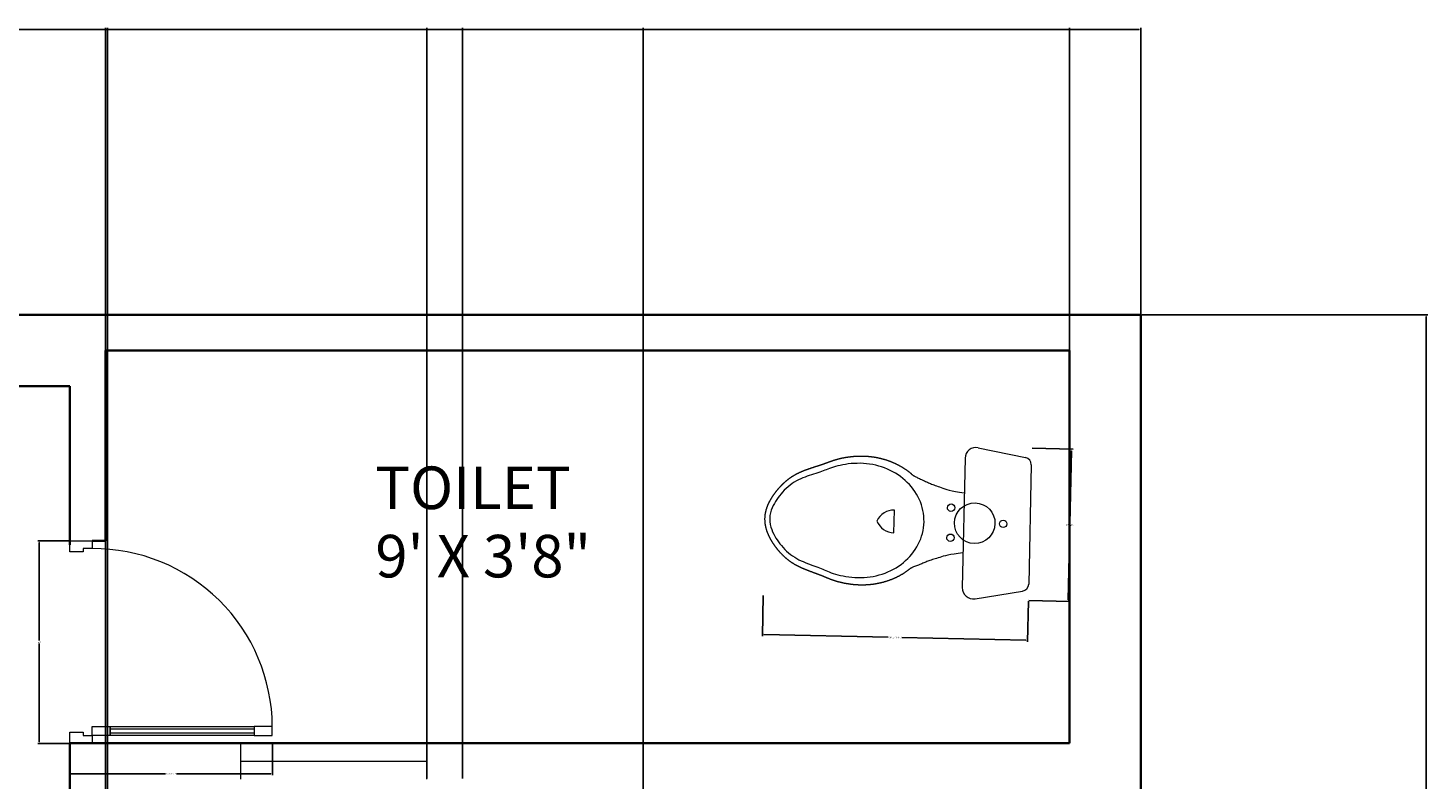
# Model space of a CAD drawing. Units: feet. Extents: x 1993 to 2298, y 2938 to 3641.
# Tile 11 of 11: x 2141 to 2298, y 3557 to 3641. Entities that reach past the tile are written whole.
import ezdxf

# ---------------------------------------------------------------- set-up
doc = ezdxf.new("R2010")
doc.units = ezdxf.units.FT
for name, color, linetype, lineweight in [('A-ANNO-DIMS', 2, 'Continuous', 18), ('A-AREA-IDEN', 7, 'Continuous', 18), ('A-DOOR', 3, 'Continuous', 18), ('A-FLOR-FIXT', 9, 'Continuous', 18), ('A-GLAZ', 4, 'Continuous', 13), ('DWV_RED', 7, 'Continuous', 0), ('WAL', 7, 'Continuous', 35)]:
    doc.layers.add(name, color=color, linetype=linetype, lineweight=lineweight)
doc.styles.get("Standard").update_dxf_attribs({"font": 'arial.ttf'})
doc.dimstyles.get("Standard").update_dxf_attribs({"dimtxt": 0.18, "dimasz": 0.18, "dimexe": 0.18, "dimexo": 0.0625, "dimgap": 0.09, "dimtad": 0, "dimtih": 1, "dimtoh": 1, "dimdec": 4, "dimzin": 0, "dimdsep": 46, "dimtxsty": 'Standard', "dimcen": 0.09, "dimadec": 0, "dimazin": 0, "dimtfac": 1, "dimtdec": 4, "dimtofl": 0, "dimtmove": 0, "dimatfit": 3, "dimfxl": 1, "dimtolj": 1, "dimtzin": 0, "dimarcsym": 0})

# ---------------------------------------------------------------- blocks, each defined once
blk = doc.blocks.new('A$C184E58E8')
for points in [[(825, 900), (825, 820), (865, 820), (865, 900)], [(825, 180), (825, 820), (865, 820), (865, 180)], [(835, 180), (835, 820), (855, 820), (855, 180)], [(825, 100), (825, 180), (865, 180), (865, 100)], [(35, 100), (35, 60), (50, 60), (50, 50), (50, 0), (0, 0), (0, 100)], [(865, 100), (900, 100), (900, 0), (850, 0), (850, 50), (850, 60), (865, 60)]]:
    blk.add_lwpolyline(points, close=True)
blk.add_arc((830, 105), 795, 90.36035, 180.36035)
blk = doc.blocks.new('A$C6F4D5F33')
at = {"layer": 'DWV_RED'}
for p, q in [((142.3, 403.6), (16.1, 380.5)), ((177.2, 29.5), (177.2, 374.6)), ((0, 42.9), (0, 361.2)), ((376.2, 337), (368.9, 333.5)), ((383.7, 340.2), (376.2, 337)), ((391.3, 343.1), (383.7, 340.2)), ((399.1, 345.6), (391.3, 343.1)), ((407, 347.8), (399.1, 345.6)), ((415, 349.7), (407, 347.8)), ((423.1, 351.2), (415, 349.7)), ((431.3, 352.5), (423.1, 351.2)), ((439.5, 353.3), (431.3, 352.5)), ((447.9, 353.8), (439.5, 353.3)), ((456.2, 354), (447.9, 353.8)), ((464.5, 353.9), (456.2, 354)), ((472.6, 353.4), (464.5, 353.9)), ((480.5, 352.6), (472.6, 353.4)), ((488.1, 351.6), (480.5, 352.6)), ((495.5, 350.4), (488.1, 351.6)), ((502.6, 349.1), (495.5, 350.4)), ((509.4, 347.5), (502.6, 349.1)), ((515.8, 345.9), (509.4, 347.5)), ((521.9, 344.1), (515.8, 345.9)), ((527.5, 342.3), (521.9, 344.1)), ((532.7, 340.4), (527.5, 342.3)), ((537.5, 338.6), (532.7, 340.4)), ((542, 336.9), (537.5, 338.6)), ((546.2, 335.2), (542, 336.9)), ((324, 300.1), (318.7, 294.3)), ((329.7, 305.8), (324, 300.1)), ((335.6, 311.2), (329.7, 305.8)), ((341.8, 316.3), (335.6, 311.2)), ((348.2, 321), (341.8, 316.3)), ((354.9, 325.5), (348.2, 321)), ((361.8, 329.7), (354.9, 325.5)), ((368.9, 333.5), (361.8, 329.7)), ((550.3, 333.5), (546.2, 335.2)), ((554.5, 331.9), (550.3, 333.5)), ((558.9, 330.3), (554.5, 331.9)), ((563.7, 328.6), (558.9, 330.3)), ((568.9, 326.8), (563.7, 328.6)), ((574.3, 324.9), (568.9, 326.8)), ((579.9, 323), (574.3, 324.9)), ((585.7, 321), (579.9, 323)), ((591.4, 318.9), (585.7, 321)), ((597.2, 316.8), (591.4, 318.9)), ((602.9, 314.5), (597.2, 316.8)), ((608.6, 312.1), (602.9, 314.5)), ((614.3, 309.5), (608.6, 312.1)), ((620, 306.6), (614.3, 309.5)), ((625.7, 303.4), (620, 306.6)), ((631.4, 299.9), (625.7, 303.4)), ((637, 296.1), (631.4, 299.9)), ((300.6, 268.4), (296.9, 261.5)), ((304.6, 275.2), (300.6, 268.4)), ((309, 281.8), (304.6, 275.2)), ((313.7, 288.1), (309, 281.8)), ((318.7, 294.3), (313.7, 288.1)), ((642.4, 291.8), (637, 296.1)), ((647.7, 287.3), (642.4, 291.8)), ((652.6, 282.7), (647.7, 287.3)), ((657.3, 277.9), (652.6, 282.7)), ((661.7, 273), (657.3, 277.9)), ((665.8, 268), (661.7, 273)), ((669.7, 263), (665.8, 268)), ((673.4, 258), (669.7, 263)), ((284.8, 224.5), (283.7, 216.9)), ((286.4, 232.1), (284.8, 224.5)), ((288.4, 239.6), (286.4, 232.1)), ((290.8, 247), (288.4, 239.6)), ((293.7, 254.3), (290.8, 247)), ((296.9, 261.5), (293.7, 254.3)), ((362.6, 232.5), (362.6, 171.6)), ((676.8, 253), (673.4, 258)), ((680.1, 247.8), (676.8, 253)), ((683.2, 242.5), (680.1, 247.8)), ((686.1, 236.7), (683.2, 242.5)), ((688.7, 230.6), (686.1, 236.7)), ((691.1, 224), (688.7, 230.6)), ((283.1, 209.2), (282.8, 201.5)), ((282.8, 201.5), (283.1, 193.8)), ((283.7, 216.9), (283.1, 209.2)), ((283.1, 193.8), (283.7, 186.1)), ((692.9, 217), (691.1, 224)), ((694.1, 209.4), (692.9, 217)), ((692.9, 186.1), (694.1, 193.6)), ((694.6, 201.5), (694.1, 209.4)), ((694.1, 193.6), (694.6, 201.5)), ((283.7, 186.1), (284.8, 178.4)), ((284.8, 178.4), (286.4, 170.8)), ((286.4, 170.8), (288.4, 163.3)), ((288.4, 163.3), (290.8, 155.9)), ((290.8, 155.9), (293.7, 148.6)), ((673.4, 145), (676.8, 150.1)), ((676.8, 150.1), (680.1, 155.2)), ((680.1, 155.2), (683.2, 160.6)), ((683.2, 160.6), (686.1, 166.3)), ((686.1, 166.3), (688.7, 172.4)), ((688.7, 172.4), (691.1, 179)), ((691.1, 179), (692.9, 186.1)), ((293.7, 148.6), (296.9, 141.5)), ((296.9, 141.5), (300.6, 134.5)), ((300.6, 134.5), (304.6, 127.7)), ((304.6, 127.7), (309, 121.2)), ((309, 121.2), (313.7, 114.8)), ((313.7, 114.8), (318.7, 108.7)), ((642.4, 111.2), (647.7, 115.7)), ((647.7, 115.7), (652.6, 120.4)), ((652.6, 120.4), (657.3, 125.2)), ((657.3, 125.2), (661.7, 130.1)), ((661.7, 130.1), (665.8, 135)), ((665.8, 135), (669.7, 140)), ((669.7, 140), (673.4, 145)), ((318.7, 108.7), (324, 102.8)), ((324, 102.8), (329.7, 97.2)), ((329.7, 97.2), (335.6, 91.8)), ((335.6, 91.8), (341.8, 86.7)), ((341.8, 86.7), (348.2, 81.9)), ((348.2, 81.9), (354.9, 77.4)), ((354.9, 77.4), (361.8, 73.3)), ((564, 74.5), (569.1, 76.3)), ((569.1, 76.3), (574.6, 78.2)), ((574.6, 78.2), (580.1, 80.1)), ((580.1, 80.1), (585.8, 82.1)), ((585.8, 82.1), (591.5, 84.2)), ((591.5, 84.2), (597.2, 86.3)), ((597.2, 86.3), (602.9, 88.6)), ((602.9, 88.6), (608.6, 91)), ((608.6, 91), (614.3, 93.6)), ((614.3, 93.6), (620, 96.4)), ((620, 96.4), (625.7, 99.6)), ((625.7, 99.6), (631.4, 103.1)), ((631.4, 103.1), (637, 107)), ((637, 107), (642.4, 111.2)), ((361.8, 73.3), (368.9, 69.4)), ((368.9, 69.4), (376.2, 65.9)), ((376.2, 65.9), (383.7, 62.7)), ((383.7, 62.7), (391.3, 59.8)), ((391.3, 59.8), (399.1, 57.3)), ((399.1, 57.3), (407, 55.1)), ((407, 55.1), (415, 53.2)), ((415, 53.2), (423.1, 51.7)), ((423.1, 51.7), (431.3, 50.5)), ((431.3, 50.5), (439.5, 49.6)), ((439.5, 49.6), (447.9, 49.1)), ((447.9, 49.1), (456.2, 48.9)), ((456.2, 48.9), (464.5, 49.1)), ((464.5, 49.1), (472.6, 49.6)), ((472.6, 49.6), (480.5, 50.3)), ((480.5, 50.3), (488.1, 51.3)), ((488.1, 51.3), (495.5, 52.5)), ((495.5, 52.5), (502.7, 53.9)), ((502.7, 53.9), (509.5, 55.4)), ((509.5, 55.4), (515.9, 57.1)), ((515.9, 57.1), (522, 58.9)), ((522, 58.9), (527.7, 60.8)), ((527.7, 60.8), (532.9, 62.6)), ((532.9, 62.6), (537.7, 64.5)), ((537.7, 64.5), (542.3, 66.2)), ((542.3, 66.2), (546.5, 68)), ((546.5, 68), (550.6, 69.6)), ((550.6, 69.6), (554.8, 71.2)), ((554.8, 71.2), (559.2, 72.8)), ((559.2, 72.8), (564, 74.5)), ((142.3, 0.5), (16.1, 23.6))]:
    blk.add_line(p, q, dxfattribs=at)
blk.add_lwpolyline([(177.2, 282.1), (189.7, 283.7), (200.3, 285.4), (209.4, 287.1), (217.2, 288.8), (223.8, 290.5), (229.5, 292.2), (234.5, 293.8), (239, 295.3), (243.3, 296.8), (247.4, 298.1), (251.3, 299.4), (254.9, 300.6), (258.4, 301.7), (261.7, 302.9), (264.8, 304), (267.8, 305.1), (270.6, 306.2), (273.3, 307.3), (275.9, 308.4), (278.5, 309.5), (281.1, 310.7), (283.7, 311.9), (286.3, 313.1), (289.1, 314.3), (291.9, 315.5), (294.8, 316.8), (297.7, 318), (300.5, 319.2), (303.3, 320.3), (305.8, 321.4), (308, 322.3), (310, 323.2), (311.5, 323.8), (312.8, 324.4), (313.8, 324.9), (314.6, 325.3), (315.2, 325.7), (315.7, 326), (316.2, 326.4), (316.7, 326.8), (317.3, 327.3), (318, 327.8), (318.7, 328.4), (319.5, 329), (320.3, 329.7), (321.1, 330.3), (322, 331), (322.9, 331.7), (323.8, 332.4), (324.7, 333.1), (325.6, 333.8), (326.5, 334.4), (327.4, 335.1), (328.3, 335.8), (329.2, 336.4), (330.1, 337.1), (331, 337.7), (331.9, 338.3), (332.9, 339), (333.8, 339.6), (334.7, 340.2), (335.7, 340.8), (336.6, 341.5), (337.6, 342.1), (338.5, 342.7), (339.5, 343.3), (340.4, 343.8), (341.4, 344.4), (342.3, 345), (343.3, 345.6), (344.3, 346.1), (345.2, 346.7), (346.2, 347.3), (347.2, 347.8), (348.2, 348.4), (349.2, 348.9), (350.2, 349.4), (351.1, 349.9), (352.1, 350.5), (353.1, 351), (354.1, 351.5), (355.1, 352), (356.2, 352.5), (357.2, 353), (358.2, 353.5), (359.2, 353.9), (360.2, 354.4), (361.2, 354.9), (362.3, 355.4), (363.3, 355.8), (364.3, 356.3), (365.4, 356.7), (366.4, 357.2), (367.4, 357.6), (368.5, 358), (369.5, 358.4), (370.6, 358.9), (371.6, 359.3), (372.7, 359.7), (373.7, 360.1), (374.8, 360.5), (375.8, 360.9), (376.9, 361.2), (378, 361.6), (379, 362), (380.1, 362.3), (381.2, 362.7), (382.3, 363.1), (383.3, 363.4), (384.4, 363.8), (385.5, 364.1), (386.6, 364.4), (387.7, 364.7), (388.7, 365.1), (389.8, 365.4), (390.9, 365.7), (392, 366), (393.1, 366.3), (394.2, 366.6), (395.3, 366.8), (396.4, 367.1), (397.5, 367.4), (398.6, 367.7), (399.7, 367.9), (400.8, 368.2), (401.9, 368.4), (403, 368.7), (404.1, 368.9), (405.2, 369.1), (406.3, 369.4), (407.4, 369.6), (408.5, 369.8), (409.7, 370), (410.8, 370.2), (411.9, 370.4), (413, 370.6), (414.1, 370.8), (415.3, 371), (416.4, 371.1), (417.5, 371.3), (418.6, 371.5), (419.8, 371.6), (420.9, 371.8), (422, 371.9), (423.1, 372.1), (424.3, 372.2), (425.4, 372.3), (426.5, 372.4), (427.7, 372.6), (428.8, 372.7), (429.9, 372.8), (431.1, 372.9), (432.2, 373), (433.4, 373.1), (434.5, 373.1), (435.6, 373.2), (436.8, 373.3), (437.9, 373.3), (439.1, 373.4), (440.2, 373.5), (441.4, 373.5), (442.5, 373.5), (443.6, 373.6), (444.8, 373.6), (445.9, 373.6), (447.1, 373.6), (448.2, 373.6), (449.3, 373.6), (450.5, 373.6), (451.6, 373.6), (452.8, 373.6), (453.9, 373.6), (455, 373.6), (456.1, 373.5), (457.3, 373.5), (458.4, 373.5), (459.5, 373.4), (460.6, 373.4), (461.7, 373.3), (462.8, 373.2), (463.9, 373.2), (465, 373.1), (466.1, 373), (467.2, 373), (468.3, 372.9), (469.4, 372.8), (470.5, 372.7), (471.5, 372.6), (472.6, 372.5), (473.7, 372.4), (474.7, 372.3), (475.8, 372.1), (476.8, 372), (477.9, 371.9), (478.9, 371.8), (480, 371.6), (481, 371.5), (482, 371.4), (483, 371.2), (484.1, 371.1), (485.1, 370.9), (486.1, 370.8), (487.1, 370.6), (488.1, 370.5), (489.1, 370.3), (490.1, 370.1), (491.1, 370), (492.1, 369.8), (493, 369.6), (494, 369.4), (495, 369.2), (495.9, 369.1), (496.9, 368.9), (497.8, 368.7), (498.8, 368.5), (499.7, 368.3), (500.7, 368.1), (501.6, 367.9), (502.5, 367.7), (503.5, 367.5), (504.4, 367.3), (505.3, 367.1), (506.2, 366.9), (507.1, 366.6), (508, 366.4), (508.9, 366.2), (509.8, 366), (510.7, 365.8), (511.5, 365.5), (512.4, 365.3), (513.3, 365.1), (514.1, 364.8), (515, 364.6), (515.8, 364.4), (516.7, 364.1), (517.5, 363.9), (518.3, 363.6), (519.1, 363.4), (519.9, 363.2), (520.7, 362.9), (521.5, 362.7), (522.3, 362.4), (523.1, 362.2), (523.9, 361.9), (524.6, 361.7), (525.4, 361.4), (526.1, 361.2), (526.9, 360.9), (527.6, 360.7), (528.3, 360.4), (529.1, 360.2), (529.8, 359.9), (530.5, 359.7), (531.2, 359.4), (531.9, 359.2), (532.5, 358.9), (533.2, 358.7), (533.9, 358.4), (534.5, 358.2), (535.2, 358), (535.8, 357.7), (536.4, 357.5), (537.1, 357.2), (537.7, 357), (538.3, 356.8), (538.9, 356.5), (539.5, 356.3), (540.1, 356.1), (540.6, 355.8), (541.2, 355.6), (541.8, 355.4), (542.3, 355.2), (542.9, 355), (543.4, 354.7), (544, 354.5), (544.5, 354.3), (545.1, 354.1), (545.6, 353.9), (546.1, 353.7), (546.6, 353.5), (547.1, 353.3), (547.6, 353.1), (548.2, 352.9), (548.7, 352.7), (549.2, 352.5), (549.6, 352.3), (550.1, 352.1), (550.6, 351.9), (551.1, 351.7), (551.6, 351.5), (552.1, 351.3), (552.6, 351.1), (553.1, 350.9), (553.6, 350.7), (554.1, 350.6), (554.6, 350.4), (555.1, 350.2), (555.6, 350), (556.1, 349.8), (556.7, 349.6), (557.2, 349.4), (557.7, 349.2), (558.3, 349), (558.8, 348.8), (559.4, 348.6), (560, 348.4), (560.5, 348.2), (561.1, 348), (561.7, 347.8), (562.3, 347.6), (562.9, 347.4), (563.5, 347.2), (564.1, 346.9), (564.7, 346.7), (565.4, 346.5), (566, 346.3), (566.6, 346.1), (567.3, 345.8), (567.9, 345.6), (568.6, 345.4), (569.2, 345.2), (569.9, 344.9), (570.6, 344.7), (571.2, 344.5), (571.9, 344.2), (572.6, 344), (573.3, 343.8), (574, 343.5), (574.7, 343.3), (575.4, 343), (576.1, 342.8), (576.8, 342.6), (577.5, 342.3), (578.2, 342.1), (578.9, 341.8), (579.6, 341.6), (580.3, 341.3), (581.1, 341.1), (581.8, 340.8), (582.5, 340.5), (583.3, 340.3), (584, 340), (584.7, 339.8), (585.4, 339.5), (586.2, 339.2), (586.9, 339), (587.7, 338.7), (588.4, 338.4), (589.1, 338.2), (589.9, 337.9), (590.6, 337.6), (591.4, 337.4), (592.1, 337.1), (592.9, 336.8), (593.6, 336.5), (594.4, 336.2), (595.1, 336), (595.9, 335.7), (596.6, 335.4), (597.4, 335.1), (598.2, 334.8), (598.9, 334.5), (599.7, 334.2), (600.4, 333.9), (601.2, 333.6), (602, 333.3), (602.7, 333), (603.5, 332.7), (604.3, 332.4), (605, 332.1), (605.8, 331.7), (606.6, 331.4), (607.3, 331.1), (608.1, 330.7), (608.9, 330.4), (609.7, 330.1), (610.5, 329.7), (611.2, 329.4), (612, 329), (612.8, 328.7), (613.6, 328.3), (614.4, 327.9), (615.2, 327.6), (616, 327.2), (616.8, 326.8), (617.6, 326.4), (618.4, 326), (619.2, 325.6), (620, 325.2), (620.8, 324.8), (621.6, 324.4), (622.4, 324), (623.2, 323.5), (624, 323.1), (624.8, 322.7), (625.6, 322.2), (626.4, 321.8), (627.2, 321.3), (628, 320.8), (628.8, 320.4), (629.6, 319.9), (630.4, 319.4), (631.2, 318.9), (632.1, 318.4), (632.9, 317.9), (633.7, 317.4), (634.5, 316.9), (635.3, 316.3), (636.1, 315.8), (636.9, 315.3), (637.7, 314.7), (638.5, 314.2), (639.3, 313.6), (640.1, 313.1), (640.9, 312.5), (641.7, 311.9), (642.5, 311.3), (643.3, 310.7), (644.1, 310.1), (644.9, 309.5), (645.7, 308.9), (646.4, 308.3), (647.2, 307.7), (648, 307.1), (648.7, 306.4), (649.5, 305.8), (650.3, 305.2), (651, 304.5), (651.8, 303.9), (652.5, 303.3), (653.2, 302.6), (654, 302), (654.7, 301.3), (655.4, 300.6), (656.1, 300), (656.8, 299.3), (657.5, 298.7), (658.2, 298), (658.9, 297.3), (659.6, 296.7), (660.2, 296), (660.9, 295.3), (661.6, 294.7), (662.2, 294), (662.9, 293.3), (663.5, 292.7), (664.2, 292), (664.8, 291.3), (665.4, 290.6), (666, 290), (666.7, 289.3), (667.3, 288.6), (667.9, 287.9), (668.5, 287.2), (669.1, 286.6), (669.7, 285.9), (670.3, 285.2), (670.9, 284.5), (671.4, 283.8), (672, 283.1), (672.6, 282.5), (673.2, 281.8), (673.7, 281.1), (674.3, 280.4), (674.8, 279.7), (675.4, 279), (675.9, 278.3), (676.5, 277.6), (677, 277), (677.5, 276.3), (678.1, 275.6), (678.6, 274.9), (679.1, 274.2), (679.6, 273.5), (680.1, 272.8), (680.6, 272.1), (681.1, 271.4), (681.6, 270.7), (682.1, 270), (682.6, 269.3), (683.1, 268.6), (683.6, 268), (684.1, 267.3), (684.5, 266.6), (685, 265.9), (685.5, 265.2), (686, 264.4), (686.4, 263.7), (686.9, 263), (687.4, 262.3), (687.8, 261.6), (688.3, 260.9), (688.7, 260.1), (689.2, 259.4), (689.6, 258.7), (690.1, 257.9), (690.5, 257.2), (691, 256.4), (691.4, 255.7), (691.9, 254.9), (692.3, 254.1), (692.7, 253.3), (693.2, 252.5), (693.6, 251.7), (694.1, 250.9), (694.5, 250.1), (694.9, 249.3), (695.3, 248.5), (695.8, 247.6), (696.2, 246.8), (696.6, 245.9), (697, 245), (697.4, 244.2), (697.8, 243.3), (698.2, 242.4), (698.6, 241.5), (699, 240.5), (699.4, 239.6), (699.8, 238.7), (700.2, 237.7), (700.6, 236.7), (700.9, 235.8), (701.3, 234.8), (701.6, 233.8), (702, 232.8), (702.3, 231.8), (702.7, 230.7), (703, 229.7), (703.3, 228.6), (703.6, 227.6), (703.9, 226.5), (704.2, 225.4), (704.5, 224.3), (704.7, 223.2), (705, 222.1), (705.2, 220.9), (705.5, 219.8), (705.7, 218.6), (705.9, 217.4), (706.1, 216.3), (706.3, 215.1), (706.4, 213.9), (706.6, 212.7), (706.7, 211.5), (706.9, 210.2), (707, 209), (707.1, 207.8), (707.1, 206.5), (707.2, 205.3), (707.2, 204), (707.3, 202.8), (707.3, 201.5), (707.3, 200.3), (707.2, 199), (707.2, 197.8), (707.1, 196.5), (707.1, 195.3), (707, 194), (706.9, 192.8), (706.7, 191.6), (706.6, 190.4), (706.4, 189.2), (706.3, 188), (706.1, 186.8), (705.9, 185.6), (705.7, 184.4), (705.5, 183.3), (705.2, 182.1), (705, 181), (704.7, 179.9), (704.5, 178.8), (704.2, 177.6), (703.9, 176.6), (703.6, 175.5), (703.3, 174.4), (703, 173.4), (702.7, 172.3), (702.3, 171.3), (702, 170.3), (701.6, 169.3), (701.3, 168.3), (700.9, 167.3), (700.6, 166.3), (700.2, 165.3), (699.8, 164.4), (699.4, 163.4), (699, 162.5), (698.6, 161.6), (698.2, 160.7), (697.8, 159.8), (697.4, 158.9), (697, 158), (696.6, 157.1), (696.2, 156.3), (695.8, 155.4), (695.3, 154.6), (694.9, 153.7), (694.5, 152.9), (694.1, 152.1), (693.6, 151.3), (693.2, 150.5), (692.7, 149.7), (692.3, 148.9), (691.9, 148.1), (691.4, 147.4), (691, 146.6), (690.5, 145.9), (690.1, 145.1), (689.6, 144.4), (689.2, 143.6), (688.7, 142.9), (688.3, 142.2), (687.8, 141.4), (687.4, 140.7), (686.9, 140), (686.4, 139.3), (686, 138.6), (685.5, 137.9), (685, 137.2), (684.5, 136.5), (684.1, 135.8), (683.6, 135.1), (683.1, 134.4), (682.6, 133.7), (682.1, 133), (681.6, 132.3), (681.1, 131.6), (680.6, 130.9), (680.1, 130.2), (679.6, 129.5), (679.1, 128.9), (678.6, 128.2), (678.1, 127.5), (677.5, 126.8), (677, 126.1), (676.5, 125.4), (675.9, 124.7), (675.4, 124), (674.8, 123.3), (674.3, 122.6), (673.7, 122), (673.2, 121.3), (672.6, 120.6), (672, 119.9), (671.4, 119.2), (670.9, 118.5), (670.3, 117.9), (669.7, 117.2), (669.1, 116.5), (668.5, 115.8), (667.9, 115.1), (667.3, 114.4), (666.7, 113.8), (666, 113.1), (665.4, 112.4), (664.8, 111.7), (664.2, 111.1), (663.5, 110.4), (662.9, 109.7), (662.2, 109), (661.6, 108.4), (660.9, 107.7), (660.2, 107), (659.6, 106.4), (658.9, 105.7), (658.2, 105), (657.5, 104.4), (656.8, 103.7), (656.1, 103.1), (655.4, 102.4), (654.7, 101.7), (654, 101.1), (653.2, 100.4), (652.5, 99.8), (651.8, 99.1), (651, 98.5), (650.3, 97.9), (649.5, 97.2), (648.7, 96.6), (648, 96), (647.2, 95.3), (646.4, 94.7), (645.7, 94.1), (644.9, 93.5), (644.1, 92.9), (643.3, 92.3), (642.5, 91.7), (641.7, 91.1), (640.9, 90.6), (640.1, 90), (639.3, 89.4), (638.5, 88.9), (637.7, 88.3), (636.9, 87.8), (636.1, 87.2), (635.3, 86.7), (634.5, 86.2), (633.7, 85.7), (632.9, 85.1), (632.1, 84.6), (631.3, 84.1), (630.4, 83.7), (629.6, 83.2), (628.8, 82.7), (628, 82.2), (627.2, 81.8), (626.4, 81.3), (625.6, 80.8), (624.8, 80.4), (624, 80), (623.2, 79.5), (622.4, 79.1), (621.6, 78.7), (620.8, 78.3), (620, 77.8), (619.2, 77.4), (618.4, 77), (617.6, 76.7), (616.8, 76.3), (616, 75.9), (615.2, 75.5), (614.4, 75.1), (613.6, 74.8), (612.8, 74.4), (612.1, 74), (611.3, 73.7), (610.5, 73.3), (609.7, 73), (608.9, 72.7), (608.2, 72.3), (607.4, 72), (606.6, 71.7), (605.8, 71.3), (605.1, 71), (604.3, 70.7), (603.5, 70.4), (602.8, 70.1), (602, 69.8), (601.3, 69.5), (600.5, 69.1), (599.7, 68.9), (599, 68.6), (598.2, 68.3), (597.5, 68), (596.7, 67.7), (596, 67.4), (595.2, 67.1), (594.5, 66.8), (593.7, 66.5), (593, 66.3), (592.2, 66), (591.5, 65.7), (590.7, 65.4), (590, 65.2), (589.3, 64.9), (588.5, 64.6), (587.8, 64.4), (587, 64.1), (586.3, 63.8), (585.6, 63.6), (584.8, 63.3), (584.1, 63.1), (583.4, 62.8), (582.7, 62.5), (581.9, 62.3), (581.2, 62), (580.5, 61.8), (579.8, 61.5), (579.1, 61.3), (578.4, 61), (577.7, 60.8), (577, 60.6), (576.3, 60.3), (575.6, 60.1), (574.9, 59.8), (574.2, 59.6), (573.5, 59.4), (572.8, 59.1), (572.1, 58.9), (571.5, 58.7), (570.8, 58.4), (570.1, 58.2), (569.5, 58), (568.8, 57.7), (568.2, 57.5), (567.5, 57.3), (566.9, 57.1), (566.2, 56.8), (565.6, 56.6), (565, 56.4), (564.4, 56.2), (563.8, 56), (563.2, 55.8), (562.6, 55.5), (562, 55.3), (561.4, 55.1), (560.8, 54.9), (560.2, 54.7), (559.7, 54.5), (559.1, 54.3), (558.6, 54.1), (558, 53.9), (557.5, 53.7), (557, 53.5), (556.5, 53.3), (555.9, 53.1), (555.4, 53), (554.9, 52.8), (554.4, 52.6), (553.9, 52.4), (553.4, 52.2), (552.9, 52), (552.4, 51.8), (551.9, 51.6), (551.5, 51.4), (551, 51.2), (550.5, 51.1), (550, 50.9), (549.5, 50.7), (549, 50.5), (548.5, 50.3), (548, 50.1), (547.5, 49.9), (546.9, 49.7), (546.4, 49.4), (545.9, 49.2), (545.4, 49), (544.8, 48.8), (544.3, 48.6), (543.8, 48.4), (543.2, 48.2), (542.6, 47.9), (542.1, 47.7), (541.5, 47.5), (540.9, 47.3), (540.4, 47), (539.8, 46.8), (539.2, 46.6), (538.6, 46.3), (538, 46.1), (537.3, 45.9), (536.7, 45.6), (536.1, 45.4), (535.4, 45.1), (534.8, 44.9), (534.1, 44.6), (533.5, 44.4), (532.8, 44.1), (532.1, 43.9), (531.4, 43.6), (530.7, 43.4), (530, 43.1), (529.3, 42.9), (528.6, 42.6), (527.8, 42.4), (527.1, 42.1), (526.4, 41.9), (525.6, 41.6), (524.8, 41.4), (524.1, 41.1), (523.3, 40.9), (522.5, 40.6), (521.7, 40.4), (520.9, 40.1), (520.1, 39.9), (519.3, 39.6), (518.5, 39.4), (517.7, 39.1), (516.8, 38.9), (516, 38.6), (515.1, 38.4), (514.3, 38.2), (513.4, 37.9), (512.5, 37.7), (511.7, 37.5), (510.8, 37.2), (509.9, 37), (509, 36.8), (508.1, 36.6), (507.2, 36.3), (506.3, 36.1), (505.4, 35.9), (504.5, 35.7), (503.6, 35.5), (502.6, 35.3), (501.7, 35.1), (500.8, 34.9), (499.8, 34.7), (498.9, 34.5), (497.9, 34.3), (497, 34.1), (496, 33.9), (495, 33.7), (494.1, 33.5), (493.1, 33.4), (492.1, 33.2), (491.1, 33), (490.1, 32.8), (489.1, 32.7), (488.1, 32.5), (487.1, 32.3), (486.1, 32.2), (485.1, 32), (484.1, 31.9), (483.1, 31.7), (482.1, 31.6), (481, 31.4), (480, 31.3), (478.9, 31.2), (477.9, 31.1), (476.9, 30.9), (475.8, 30.8), (474.7, 30.7), (473.7, 30.6), (472.6, 30.5), (471.6, 30.4), (470.5, 30.3), (469.4, 30.2), (468.3, 30.1), (467.2, 30), (466.1, 29.9), (465, 29.8), (463.9, 29.8), (462.8, 29.7), (461.7, 29.6), (460.6, 29.6), (459.5, 29.5), (458.4, 29.5), (457.3, 29.4), (456.1, 29.4), (455, 29.4), (453.9, 29.3), (452.8, 29.3), (451.6, 29.3), (450.5, 29.3), (449.3, 29.3), (448.2, 29.3), (447.1, 29.3), (445.9, 29.3), (444.8, 29.3), (443.6, 29.4), (442.5, 29.4), (441.4, 29.4), (440.2, 29.5), (439.1, 29.5), (437.9, 29.6), (436.8, 29.7), (435.6, 29.7), (434.5, 29.8), (433.4, 29.9), (432.2, 30), (431.1, 30.1), (429.9, 30.2), (428.8, 30.3), (427.7, 30.4), (426.5, 30.5), (425.4, 30.6), (424.3, 30.7), (423.1, 30.9), (422, 31), (420.9, 31.2), (419.8, 31.3), (418.6, 31.5), (417.5, 31.6), (416.4, 31.8), (415.3, 32), (414.1, 32.2), (413, 32.3), (411.9, 32.5), (410.8, 32.7), (409.7, 32.9), (408.5, 33.1), (407.4, 33.4), (406.3, 33.6), (405.2, 33.8), (404.1, 34), (403, 34.3), (401.9, 34.5), (400.8, 34.8), (399.7, 35), (398.6, 35.3), (397.5, 35.5), (396.4, 35.8), (395.3, 36.1), (394.2, 36.4), (393.1, 36.7), (392, 37), (390.9, 37.3), (389.8, 37.6), (388.7, 37.9), (387.7, 38.2), (386.6, 38.5), (385.5, 38.9), (384.4, 39.2), (383.3, 39.5), (382.3, 39.9), (381.2, 40.2), (380.1, 40.6), (379, 41), (378, 41.3), (376.9, 41.7), (375.8, 42.1), (374.8, 42.5), (373.7, 42.9), (372.7, 43.3), (371.6, 43.7), (370.6, 44.1), (369.5, 44.5), (368.5, 44.9), (367.4, 45.4), (366.4, 45.8), (365.4, 46.2), (364.3, 46.7), (363.3, 47.1), (362.3, 47.6), (361.2, 48), (360.2, 48.5), (359.2, 49), (358.2, 49.5), (357.2, 50), (356.2, 50.5), (355.1, 50.9), (354.1, 51.5), (353.1, 52), (352.1, 52.5), (351.1, 53), (350.2, 53.5), (349.2, 54.1), (348.2, 54.6), (347.2, 55.1), (346.2, 55.7), (345.2, 56.2), (344.3, 56.8), (343.3, 57.4), (342.3, 57.9), (341.4, 58.5), (340.4, 59.1), (339.5, 59.7), (338.5, 60.3), (337.6, 60.9), (336.6, 61.5), (335.7, 62.1), (334.7, 62.7), (333.8, 63.3), (332.9, 64), (331.9, 64.6), (331, 65.2), (330.1, 65.9), (329.2, 66.5), (328.3, 67.2), (327.4, 67.8), (326.5, 68.5), (325.6, 69.2), (324.7, 69.9), (323.8, 70.5), (322.9, 71.2), (322, 71.9), (321.1, 72.6), (320.3, 73.3), (319.5, 74), (318.7, 74.6), (317.9, 75.3), (317.2, 75.9), (316.5, 76.4), (315.9, 76.9), (315.3, 77.4), (314.6, 77.9), (313.9, 78.5), (313, 79), (311.9, 79.6), (310.6, 80.3), (309, 81.1), (307.1, 82), (304.9, 82.9), (302.5, 84), (299.9, 85.1), (297.2, 86.3), (294.4, 87.5), (291.6, 88.7), (288.8, 89.9), (286.2, 91.1), (283.6, 92.3), (281, 93.4), (278.5, 94.6), (275.9, 95.7), (273.3, 96.8), (270.6, 97.9), (267.8, 99), (264.8, 100.1), (261.7, 101.2), (258.4, 102.4), (254.9, 103.5), (251.3, 104.7), (247.4, 106), (243.3, 107.3), (239, 108.8), (234.5, 110.3), (229.5, 111.9), (223.8, 113.6), (217.2, 115.3), (209.4, 117), (200.3, 118.7), (189.7, 120.4), (177.2, 122)], dxfattribs=at)
for centre, major_axis, start_param, end_param in [((19.7, 361.2), (-13.9, 13.9), 5.678651, 7.068583), ((147.6, 374.6), (-20.9, 20.9), 3.926991, 5.678651), ((147.6, 202.1), (-38.3, 38.3), 0.785398, 7.068583), ((211.6, 242.1), (-6.96, 6.96), 0.785398, 7.068583), ((362.6, 182.9), (-35.1, -35.1), 2.753037, 3.926991), ((71.5, 202.2), (-6.96, -6.96), -0.785398, 5.497787), ((362.6, 221.2), (-35.1, 35.1), 2.356194, 3.530149), ((211.6, 162), (-6.96, 6.96), 0.785398, 7.068583), ((19.7, 42.9), (-13.9, -13.9), -0.785398, 0.604534), ((147.6, 29.5), (-20.9, -20.9), 0.604534, 2.356194)]:
    blk.add_ellipse(centre, major_axis=major_axis, ratio=1, start_param=start_param, end_param=end_param, dxfattribs=at)
blk = doc.blocks.new('*D22')
at = {"layer": 'A-ANNO-DIMS', "color": 0, "lineweight": -2, "transparency": 16777216}
for p, q in [((2145.76, 3560.47), (2145.76, 3556.95)), ((2168.46, 3560.47), (2168.46, 3556.95)), ((2145.94, 3557.13), (2156.48, 3557.13)), ((2168.28, 3557.13), (2157.74, 3557.13))]:
    blk.add_line(p, q, dxfattribs=at)
at = {"layer": 'A-ANNO-DIMS', "color": 0, "transparency": 16777216}
for points in [[(2145.94, 3557.16), (2145.94, 3557.1), (2145.76, 3557.13)], [(2168.28, 3557.16), (2168.28, 3557.1), (2168.46, 3557.13)]]:
    blk.add_solid(points, dxfattribs=at)
at = {"layer": 'Defpoints', "color": 0, "transparency": 16777216}
for p in [(2145.76, 3560.53), (2168.46, 3560.53), (2168.46, 3557.13)]:
    blk.add_point(p, dxfattribs=at)
at = {"layer": 'A-ANNO-DIMS', "color": 0, "transparency": 16777216, "insert": (2157.11, 3557.13), "char_height": 0.18, "attachment_point": 5}
blk.add_mtext('\\A1;DOOR 23', dxfattribs=at)
blk = doc.blocks.new('*D23')
at = {"layer": 'A-ANNO-DIMS', "color": 0, "lineweight": -2, "transparency": 16777216}
for p, q in [((2145.7, 3583.23), (2142.17, 3583.23)), ((2142.35, 3583.05), (2142.35, 3572.07)), ((2142.35, 3560.71), (2142.35, 3571.7)), ((2145.7, 3560.53), (2142.17, 3560.53))]:
    blk.add_line(p, q, dxfattribs=at)
at = {"layer": 'A-ANNO-DIMS', "color": 0, "transparency": 16777216}
for points in [[(2142.32, 3583.05), (2142.38, 3583.05), (2142.35, 3583.23)], [(2142.32, 3560.71), (2142.38, 3560.71), (2142.35, 3560.53)]]:
    blk.add_solid(points, dxfattribs=at)
at = {"layer": 'Defpoints', "color": 0, "transparency": 16777216}
for p in [(2145.76, 3583.23), (2142.35, 3560.53), (2145.76, 3560.53)]:
    blk.add_point(p, dxfattribs=at)
at = {"layer": 'A-ANNO-DIMS', "color": 0, "transparency": 16777216, "insert": (2142.35, 3571.88), "char_height": 0.18, "attachment_point": 5}
blk.add_mtext('\\A1;23', dxfattribs=at)
blk = doc.blocks.new('*D32')
at = {"layer": 'A-ANNO-DIMS', "color": 0, "lineweight": -2, "transparency": 16777216}
for p, q in [((2223.46, 3577.11), (2223.36, 3572.54)), ((2253.16, 3576.47), (2253.06, 3571.9)), ((2223.54, 3572.71), (2237.44, 3572.41)), ((2252.88, 3572.08), (2238.99, 3572.38))]:
    blk.add_line(p, q, dxfattribs=at)
at = {"layer": 'A-ANNO-DIMS', "color": 0, "transparency": 16777216}
for points in [[(2223.54, 3572.74), (2223.54, 3572.68), (2223.36, 3572.72)], [(2252.88, 3572.11), (2252.88, 3572.05), (2253.06, 3572.08)]]:
    blk.add_solid(points, dxfattribs=at)
at = {"layer": 'Defpoints', "color": 0, "transparency": 16777216}
for p in [(2223.46, 3577.17), (2253.16, 3576.53), (2223.36, 3572.72)]:
    blk.add_point(p, dxfattribs=at)
at = {"layer": 'A-ANNO-DIMS', "color": 0, "transparency": 16777216, "insert": (2238.21, 3572.4), "char_height": 0.18, "attachment_point": 5}
blk.add_mtext('\\A1;WC 30 TYP.', dxfattribs=at)
blk = doc.blocks.new('*D33')
at = {"layer": 'A-ANNO-DIMS', "color": 0, "lineweight": -2, "transparency": 16777216}
for p, q in [((2253.59, 3593.59), (2258.16, 3593.49)), ((2257.98, 3593.31), (2257.8, 3585.15)), ((2257.62, 3576.62), (2257.79, 3584.78)), ((2253.22, 3576.53), (2257.79, 3576.43))]:
    blk.add_line(p, q, dxfattribs=at)
at = {"layer": 'A-ANNO-DIMS', "color": 0, "transparency": 16777216}
for points in [[(2257.95, 3593.31), (2258.01, 3593.31), (2257.98, 3593.49)], [(2257.59, 3576.62), (2257.65, 3576.62), (2257.61, 3576.44)]]:
    blk.add_solid(points, dxfattribs=at)
at = {"layer": 'Defpoints', "color": 0, "transparency": 16777216}
for p in [(2253.52, 3593.59), (2253.16, 3576.53), (2257.61, 3576.44)]:
    blk.add_point(p, dxfattribs=at)
at = {"layer": 'A-ANNO-DIMS', "color": 0, "transparency": 16777216, "insert": (2257.8, 3584.97), "char_height": 0.18, "attachment_point": 5}
blk.add_mtext('\\A1;17 TYP.', dxfattribs=at)
blk = doc.blocks.new('*D54')
at = {"layer": 'A-ANNO-DIMS', "color": 0, "lineweight": -2, "transparency": 16777216}
for p, q in [((2025.76, 3608.6), (2025.76, 3640.68)), ((2025.94, 3640.5), (2145.47, 3640.5)), ((2265.58, 3640.5), (2146.05, 3640.5)), ((2265.76, 3608.6), (2265.76, 3640.68))]:
    blk.add_line(p, q, dxfattribs=at)
at = {"layer": 'A-ANNO-DIMS', "color": 0, "transparency": 16777216}
for points in [[(2025.94, 3640.53), (2025.94, 3640.47), (2025.76, 3640.5)], [(2265.58, 3640.53), (2265.58, 3640.47), (2265.76, 3640.5)]]:
    blk.add_solid(points, dxfattribs=at)
at = {"layer": 'Defpoints', "color": 0, "transparency": 16777216}
for p in [(2265.76, 3640.5), (2025.76, 3608.53), (2265.76, 3608.53)]:
    blk.add_point(p, dxfattribs=at)
at = {"layer": 'A-ANNO-DIMS', "color": 0, "transparency": 16777216, "insert": (2145.76, 3640.5), "char_height": 0.18, "attachment_point": 5}
blk.add_mtext('\\A1;240', dxfattribs=at)
blk = doc.blocks.new('*D55')
at = {"layer": 'A-ANNO-DIMS', "color": 0, "lineweight": -2, "transparency": 16777216}
for p, q in [((2265.82, 3608.53), (2297.9, 3608.53)), ((2297.72, 3608.35), (2297.72, 3308.72)), ((2297.72, 3008.71), (2297.72, 3308.35)), ((2265.82, 3008.53), (2297.9, 3008.53))]:
    blk.add_line(p, q, dxfattribs=at)
at = {"layer": 'A-ANNO-DIMS', "color": 0, "transparency": 16777216}
for points in [[(2297.69, 3608.35), (2297.75, 3608.35), (2297.72, 3608.53)], [(2297.69, 3008.71), (2297.75, 3008.71), (2297.72, 3008.53)]]:
    blk.add_solid(points, dxfattribs=at)
at = {"layer": 'Defpoints', "color": 0, "transparency": 16777216}
for p in [(2265.76, 3608.53), (2297.72, 3608.53), (2265.76, 3008.53)]:
    blk.add_point(p, dxfattribs=at)
at = {"layer": 'A-ANNO-DIMS', "color": 0, "transparency": 16777216, "insert": (2297.72, 3308.53), "char_height": 0.18, "attachment_point": 5}
blk.add_mtext('\\A1;600', dxfattribs=at)
blk = doc.blocks.new('*D59')
at = {"layer": 'A-ANNO-DIMS', "color": 0, "lineweight": -2, "transparency": 16777216}
for p, q in [((2140, 3048.6), (2140, 3640.68)), ((2140.18, 3640.5), (2144.79, 3640.5)), ((2149.82, 3640.5), (2145.21, 3640.5)), ((2150, 3048.6), (2150, 3640.68))]:
    blk.add_line(p, q, dxfattribs=at)
at = {"layer": 'A-ANNO-DIMS', "color": 0, "transparency": 16777216}
for points in [[(2140.18, 3640.53), (2140.18, 3640.47), (2140, 3640.5)], [(2149.82, 3640.53), (2149.82, 3640.47), (2150, 3640.5)]]:
    blk.add_solid(points, dxfattribs=at)
at = {"layer": 'Defpoints', "color": 0, "transparency": 16777216}
for p in [(2150, 3640.5), (2140, 3048.53), (2150, 3048.53)]:
    blk.add_point(p, dxfattribs=at)
at = {"layer": 'A-ANNO-DIMS', "color": 0, "transparency": 16777216, "insert": (2145, 3640.5), "char_height": 0.18, "attachment_point": 5}
blk.add_mtext('\\A1;10', dxfattribs=at)
blk = doc.blocks.new('*D63')
at = {"layer": 'A-ANNO-DIMS', "color": 0, "lineweight": -2, "transparency": 16777216}
for p, q in [((2257.76, 3604.6), (2257.76, 3640.68)), ((2257.94, 3640.5), (2261.61, 3640.5)), ((2265.58, 3640.5), (2261.91, 3640.5)), ((2265.76, 3608.6), (2265.76, 3640.68))]:
    blk.add_line(p, q, dxfattribs=at)
at = {"layer": 'A-ANNO-DIMS', "color": 0, "transparency": 16777216}
for points in [[(2257.94, 3640.53), (2257.94, 3640.47), (2257.76, 3640.5)], [(2265.58, 3640.53), (2265.58, 3640.47), (2265.76, 3640.5)]]:
    blk.add_solid(points, dxfattribs=at)
at = {"layer": 'Defpoints', "color": 0, "transparency": 16777216}
for p in [(2265.76, 3640.5), (2265.76, 3608.53), (2257.76, 3604.53)]:
    blk.add_point(p, dxfattribs=at)
at = {"layer": 'A-ANNO-DIMS', "color": 0, "transparency": 16777216, "insert": (2261.76, 3640.5), "char_height": 0.18, "attachment_point": 5}
blk.add_mtext('\\A1;8', dxfattribs=at)
blk = doc.blocks.new('*D64')
at = {"layer": 'A-ANNO-DIMS', "color": 0, "lineweight": -2, "transparency": 16777216}
for p, q in [((2185.76, 3556.6), (2185.76, 3640.68)), ((2185.94, 3640.5), (2187.61, 3640.5)), ((2189.58, 3640.5), (2187.91, 3640.5)), ((2189.76, 3556.6), (2189.76, 3640.68))]:
    blk.add_line(p, q, dxfattribs=at)
at = {"layer": 'A-ANNO-DIMS', "color": 0, "transparency": 16777216}
for points in [[(2185.94, 3640.53), (2185.94, 3640.47), (2185.76, 3640.5)], [(2189.58, 3640.53), (2189.58, 3640.47), (2189.76, 3640.5)]]:
    blk.add_solid(points, dxfattribs=at)
at = {"layer": 'Defpoints', "color": 0, "transparency": 16777216}
for p in [(2189.76, 3640.5), (2185.76, 3556.53), (2189.76, 3556.53)]:
    blk.add_point(p, dxfattribs=at)
at = {"layer": 'A-ANNO-DIMS', "color": 0, "transparency": 16777216, "insert": (2187.76, 3640.5), "char_height": 0.18, "attachment_point": 5}
blk.add_mtext('\\A1;4', dxfattribs=at)
blk = doc.blocks.new('*D73')
at = {"layer": 'A-ANNO-DIMS', "color": 0, "lineweight": -2, "transparency": 16777216}
for p, q in [((2149.76, 3105.6), (2149.76, 3640.68)), ((2149.94, 3640.5), (2179.49, 3640.5)), ((2209.82, 3640.5), (2180.27, 3640.5)), ((2210, 3105.6), (2210, 3640.68))]:
    blk.add_line(p, q, dxfattribs=at)
at = {"layer": 'A-ANNO-DIMS', "color": 0, "transparency": 16777216}
for points in [[(2149.94, 3640.53), (2149.94, 3640.47), (2149.76, 3640.5)], [(2209.82, 3640.53), (2209.82, 3640.47), (2210, 3640.5)]]:
    blk.add_solid(points, dxfattribs=at)
at = {"layer": 'Defpoints', "color": 0, "transparency": 16777216}
for p in [(2210, 3640.5), (2149.76, 3105.53), (2210, 3105.53)]:
    blk.add_point(p, dxfattribs=at)
at = {"layer": 'A-ANNO-DIMS', "color": 0, "transparency": 16777216, "insert": (2179.88, 3640.5), "char_height": 0.18, "attachment_point": 5}
blk.add_mtext('\\A1;60.24', dxfattribs=at)

msp = doc.modelspace()

# ---------------------------------------------------------------- linework, layer by layer
at = {"layer": 'A-GLAZ'}
for p, q in [((2164.9041, 3560.5338), (2164.9041, 3556.5338)), ((2185.7583, 3556.5338), (2185.7583, 3560.5338)), ((2164.9041, 3558.5338), (2185.7583, 3558.5338))]:
    msp.add_line(p, q, dxfattribs=at)
at = {"layer": 'WAL'}
for p, q in [((2025.7583, 3608.5338), (2265.7583, 3608.5338)), ((2265.7583, 3608.5338), (2265.7583, 3008.5338)), ((2149.7583, 3604.5338), (2257.7583, 3604.5338)), ((2149.7583, 3584.5338), (2149.7583, 3604.5338)), ((2257.7583, 3604.5338), (2257.7583, 3560.5338)), ((2033.7583, 3600.5338), (2145.7583, 3600.5338)), ((2145.7583, 3584.5338), (2145.7583, 3600.5338)), ((2145.7583, 3584.5338), (2145.7583, 3582.7601)), ((2149.7583, 3583.2341), (2149.7583, 3584.5338)), ((2148.2806, 3583.2341), (2149.7583, 3583.2341)), ((2145.7583, 3560.5338), (2257.7583, 3560.5338)), ((2145.7583, 3432.5338), (2145.7583, 3560.5338))]:
    msp.add_line(p, q, dxfattribs=at)

# ---------------------------------------------------------------- block references
at = {"layer": 'A-DOOR', "xscale": 0.0252225346102042, "yscale": 0.0252225346102042, "zscale": 0.0252225346102042, "rotation": 270}
msp.add_blockref('A$C184E58E8', (2145.7583, 3583.2341), dxfattribs=at)
at = {"layer": 'A-FLOR-FIXT', "xscale": 0.0419889779106581, "yscale": 0.0419889779106581, "zscale": 0.0419889779106581, "rotation": 178.7655746873133}
msp.add_blockref('A$C6F4D5F33', (2253.5239, 3593.5429), dxfattribs=at)

# ---------------------------------------------------------------- texts
at = {"layer": 'A-AREA-IDEN'}
for s, p in [('TOILET', (2180, 3586.7773)), ('9\' X 3\'8"', (2180, 3579.1194))]:
    msp.add_text(s, height=4.76705, dxfattribs=at).set_placement(p)

# ---------------------------------------------------------------- dimensions: what is measured, and where the dimension line sits
at = {"layer": 'A-ANNO-DIMS'}
for base, p1, p2, override, picture, middle in [((2265.7583, 3640.4988), (2025.7583, 3608.5338), (2265.7583, 3608.5338), {"dimdec": 0, "dimlfac": 1, "dimrnd": 0, "dimzin": 0, "dimdsep": 46, "dimlunit": 2}, '*D54', (2145.7583, 3640.4988)), ((2150, 3640.4988), (2140, 3048.5338), (2150, 3048.5338), {"dimdec": 0, "dimlfac": 1, "dimrnd": 0, "dimzin": 0, "dimdsep": 46, "dimlunit": 2}, '*D59', (2145, 3640.4988)), ((2210, 3640.4988), (2149.7583, 3105.5338), (2210, 3105.5338), {"dimdec": 2, "dimlfac": 1, "dimrnd": 0, "dimzin": 0, "dimdsep": 46, "dimlunit": 2}, '*D73', (2179.8792, 3640.4988)), ((2189.7583, 3640.4988), (2185.7583, 3556.5338), (2189.7583, 3556.5338), {"dimdec": 0, "dimlfac": 1, "dimrnd": 0, "dimzin": 0, "dimdsep": 46, "dimlunit": 2}, '*D64', (2187.7583, 3640.4988)), ((2265.7583, 3640.4988), (2257.7583, 3604.5338), (2265.7583, 3608.5338), {"dimdec": 0, "dimlfac": 1, "dimrnd": 0, "dimzin": 0, "dimdsep": 46, "dimlunit": 2}, '*D63', (2261.7583, 3640.4988))]:
    dim = msp.add_linear_dim(base=base, p1=p1, p2=p2, dimstyle='Standard', override=override, dxfattribs=at)
    dim.commit()
    dim.dimension.update_dxf_attribs({"geometry": picture, "text_midpoint": middle})
for base, p1, p2, angle, picture, middle in [((2297.7233, 3608.5338), (2265.7583, 3008.5338), (2265.7583, 3608.5338), 90, '*D55', (2297.7233, 3308.5338)), ((2142.3533, 3560.5338), (2145.7583, 3583.2341), (2145.7583, 3560.5338), 270, '*D23', (2142.3533, 3571.8839))]:
    dim = msp.add_linear_dim(base=base, p1=p1, p2=p2, angle=angle, dimstyle='Standard', override={"dimdec": 0, "dimlfac": 1, "dimrnd": 0, "dimzin": 0, "dimdsep": 46, "dimlunit": 2}, dxfattribs=at)
    dim.commit()
    dim.dimension.update_dxf_attribs({"geometry": picture, "text_midpoint": middle})
for base, p1, p2, angle, text, picture, middle in [((2257.6121, 3576.437), (2253.5249, 3593.589), (2253.1574, 3576.533), 268.765575, '<> TYP.', '*D33', (2257.7959, 3584.965)), ((2223.3627, 3572.7182), (2253.1574, 3576.533), (2223.4587, 3577.173), 178.765575, 'WC <> TYP.', '*D32', (2238.212, 3572.3982))]:
    dim = msp.add_linear_dim(base=base, p1=p1, p2=p2, angle=angle, text=text, dimstyle='Standard', override={"dimdec": 0, "dimlfac": 1, "dimrnd": 0, "dimzin": 0, "dimdsep": 46, "dimlunit": 2}, dxfattribs=at)
    dim.commit()
    dim.dimension.update_dxf_attribs({"geometry": picture, "text_midpoint": middle})
dim = msp.add_linear_dim(base=(2168.4586, 3557.1288), p1=(2145.7583, 3560.5338), p2=(2168.4586, 3560.5338), text='DOOR <>', dimstyle='Standard', override={"dimdec": 0, "dimlfac": 1, "dimrnd": 0, "dimzin": 0, "dimdsep": 46, "dimlunit": 2}, dxfattribs=at)
dim.commit()
dim.dimension.update_dxf_attribs({"geometry": '*D22', "text_midpoint": (2157.1085, 3557.1288)})

doc.saveas('drawing.dxf')
